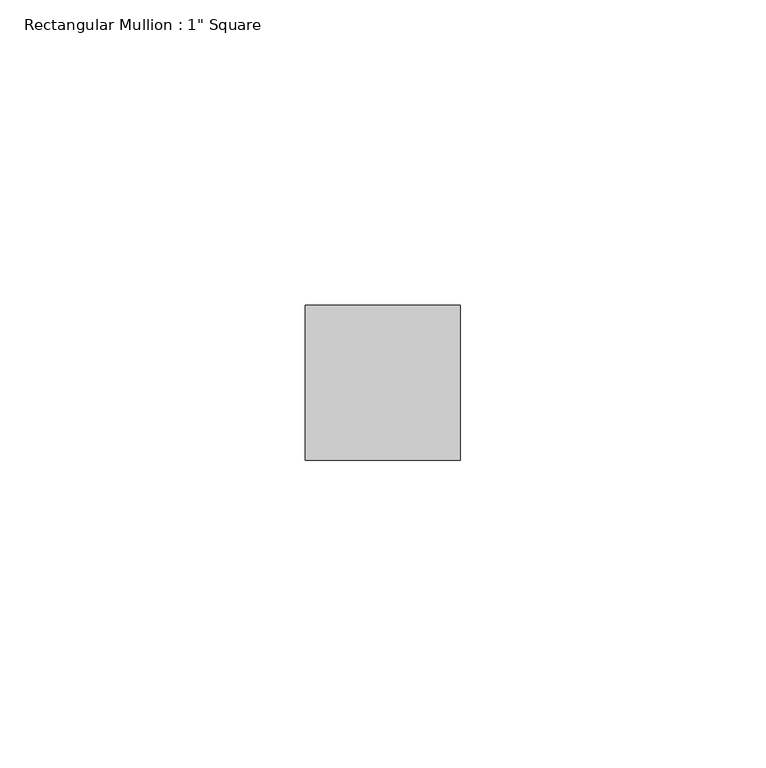
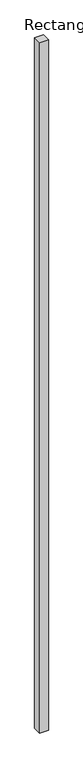
"""IFC4 building model written with IfcOpenShell, lengths in millimetres: member geometry."""

from ifc_helpers import new_model, si_unit, frame, origin, place, context, project, spatial, polyline, outline, extrude, source, transform, mapped, element, save


def member_90203b35(model_context):
    return source(origin(), model_context, "Body", "SweptSolid", [
        extrude(outline(polyline([(0.0, 12.7), (0.0, -12.7), (-25.4, -12.7), (-25.4, 12.7), (0.0, 12.7)])), frame((0.0, 0.0, -2139.95), z_axis=(0.0, 0.0, 1.0), x_axis=(1.0, 0.0, 0.0)), (0.0, 0.0, 1.0), 2139.95),
    ])


if __name__ == "__main__":
    model = new_model("IFC4")
    model_context = context("Model", 3, world=origin())
    ifc_project = project(units=[si_unit("LENGTHUNIT", "METRE", prefix="MILLI")], contexts=[model_context])
    site = spatial("IfcSite", under=ifc_project)
    building = spatial("IfcBuilding", under=site)
    placement = place(None, origin())
    member_shape = member_90203b35(model_context)
    element("IfcMember", 1, ObjectType="Rectangular Mullion : 1\" Square", at=placement, inside=building, context=model_context, shape_type="MappedRepresentation", body=[
        mapped(member_shape, transform((0.0, 0.0, 0.0), x_axis=(1.0, 0.0, 0.0), y_axis=(0.0, 1.0, 0.0), z_axis=(0.0, 0.0, 1.0))),
    ])
    save(model, "model.ifc")

# Revit data of these elements
# Type "Rectangular Mullion : 1\" Square"
#   built-in parameter 1007304 = 0.0833333 (stored number, unit not read)
#   built-in parameter 1007301 = 0.0416667 (stored number, unit not read)
#   built-in parameter 1007300 = 0.0416667 (stored number, unit not read)
# Element 1 (IfcMember, "Rectangular Mullion : 1\" Square")
#   Materials on its faces: "Aluminum"
# Materials
#   "Aluminum": class "Metal", colour RGB 247 247 247, transparency 0, Description = "Aluminum 6061", Cost = 0
